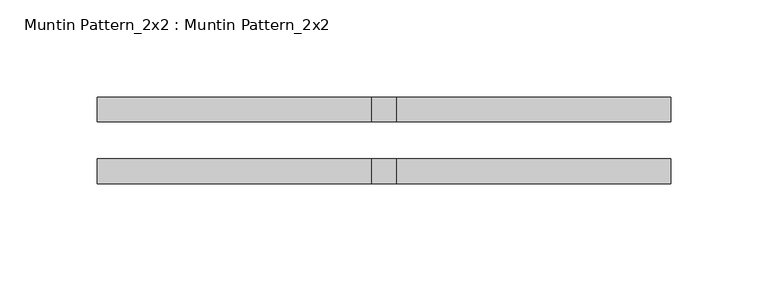
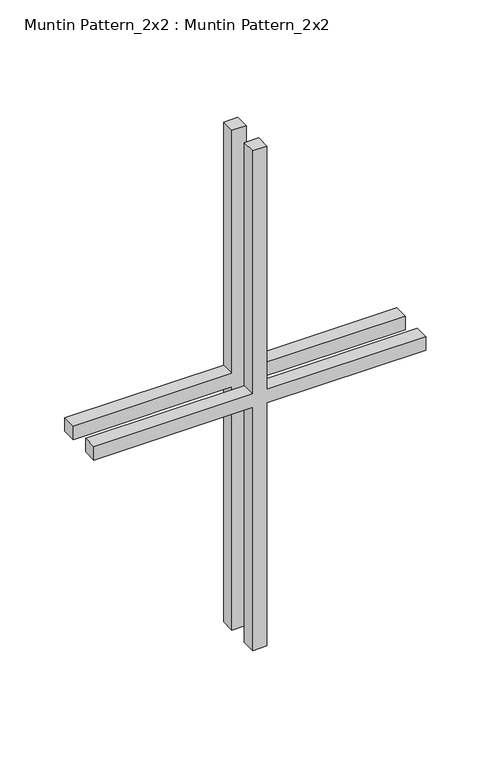
"""IFC4 building model written with IfcOpenShell, lengths in millimetres: proxy geometry, Muntin Pattern_2x2 : Muntin Pattern_2x2."""

from ifc_helpers import new_model, si_unit, frame, origin, place, context, project, spatial, polyline, outline, extrude, source, transform, mapped, element, save


def muntin_pattern_2x2_muntin_pattern_2x2_27bf4e5b(model_context):
    return source(origin(), model_context, "Body", "SweptSolid", [
        extrude(outline(polyline([(241.3, -6.35), (241.3, -147.6375), (228.6, -147.6375), (228.6, -6.35), (0.0, -6.35), (0.0, 6.35), (228.6, 6.35), (228.6, 147.6375), (241.3, 147.6375), (241.3, 6.35), (469.9, 6.35), (469.9, -6.35), (241.3, -6.35)])), frame((0.0, -22.225, 0.0), z_axis=(0.0, 1.0, 0.0), x_axis=(0.0, 0.0, 1.0)), (0.0, 0.0, 1.0), 12.7),
        extrude(outline(polyline([(241.3, -6.35), (241.3, -147.6375), (228.6, -147.6375), (228.6, -6.35), (0.0, -6.35), (0.0, 6.35), (228.6, 6.35), (228.6, 147.6375), (241.3, 147.6375), (241.3, 6.35), (469.9, 6.35), (469.9, -6.35), (241.3, -6.35)])), frame((0.0, 9.525, 0.0), z_axis=(0.0, 1.0, 0.0), x_axis=(0.0, 0.0, 1.0)), (0.0, 0.0, 1.0), 12.7),
    ])


if __name__ == "__main__":
    model = new_model("IFC4")
    model_context = context("Model", 3, world=origin())
    ifc_project = project(units=[si_unit("LENGTHUNIT", "METRE", prefix="MILLI")], contexts=[model_context])
    site = spatial("IfcSite", under=ifc_project)
    building = spatial("IfcBuilding", under=site)
    placement = place(None, origin())
    muntin_pattern_2x2_muntin_pattern_2x2_shape = muntin_pattern_2x2_muntin_pattern_2x2_27bf4e5b(model_context)
    element("IfcBuildingElementProxy", 1, Name="Muntin Pattern_2x2 : Muntin Pattern_2x2", ObjectType="Muntin Pattern_2x2 : Muntin Pattern_2x2", at=placement, inside=building, context=model_context, shape_type="MappedRepresentation", body=[
        mapped(muntin_pattern_2x2_muntin_pattern_2x2_shape, transform((0.0, 0.0, 0.0), x_axis=(1.0, 0.0, 0.0), y_axis=(0.0, 1.0, 0.0), z_axis=(0.0, 0.0, 1.0))),
    ])
    save(model, "model.ifc")

# Revit data of these elements
# Type "Muntin Pattern_2x2 : Muntin Pattern_2x2"
#   Width [instance default] = 4' - 0"
#   Thickness = 0' - 0 1/2"
#   Height [instance default] = 4' - 0"
#   Distance = 0' - 0 3/4"
#   Interior Material [instance default] = none
#   Exterior Material [instance default] = none
#   Default Elevation = 0
# Element 1 (IfcBuildingElementProxy, "Muntin Pattern_2x2 : Muntin Pattern_2x2")
#   Width = 0' - 11 5/8"
#   Height = 1' - 6 1/2"
#   Interior Material = Wood - Stained
#   Exterior Material = Clad - White
#   Materials on its faces: "Clad - White", "Wood - Stained"
# Materials
#   "Clad - White": class "Wood", colour RGB 242 242 238, transparency 0, Cost = 0
#   "Wood - Stained": class "Wood", colour RGB 224 178 126, transparency 0, Cost = 0
